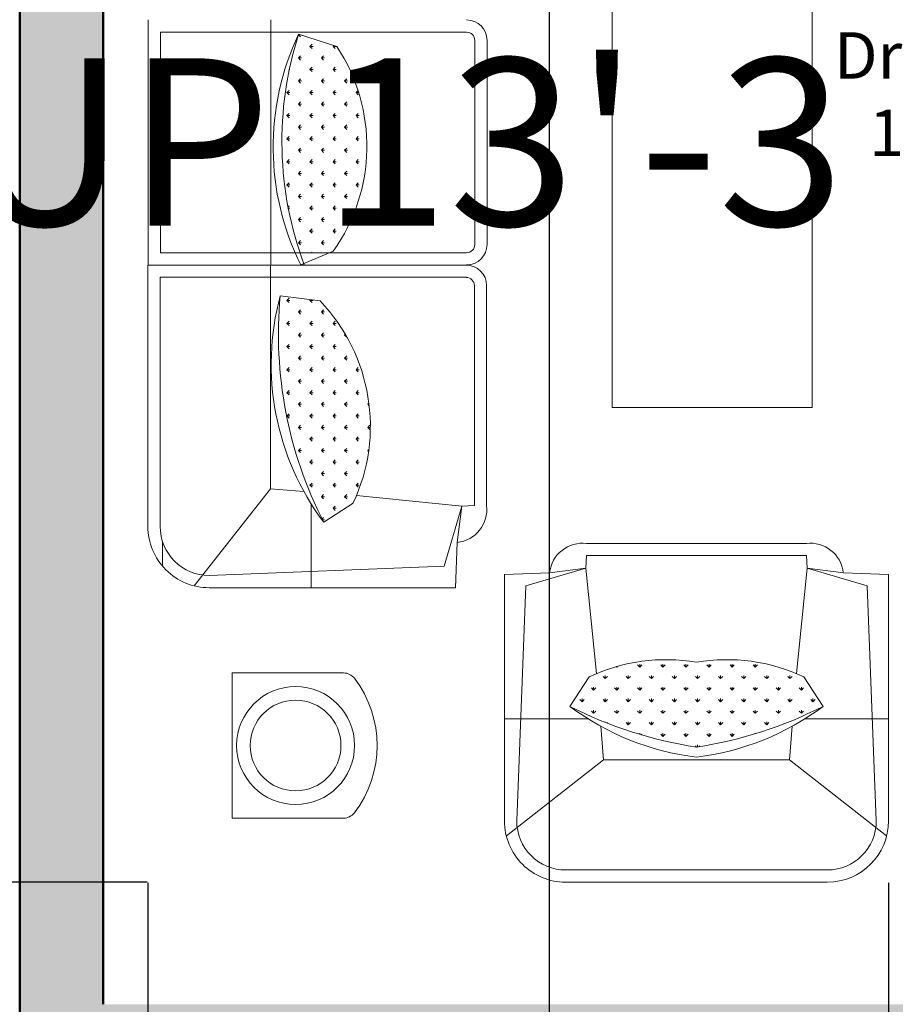
# Model space of a CAD drawing. Units: inches. Extents: x 2796 to 3603, y 978 to 1787.
# Tile 3 of 15: x 3070 to 3165, y 1116 to 1222. Entities that reach past the tile are written whole.
import ezdxf

# ---------------------------------------------------------------- set-up
doc = ezdxf.new("R2010")
doc.units = ezdxf.units.IN
for name, color, linetype, lineweight in [('A-ANNO-DIMS', 7, 'Continuous', 18), ('A-AREA-IDEN', 7, 'Continuous', 18), ('A-WALL-EXTR-PATT', 1, 'Continuous', 13), ('Furniture', 2, 'Continuous', 18), ('Outer Wall', 1, 'Continuous', 50)]:
    doc.layers.add(name, color=color, linetype=linetype, lineweight=lineweight)
doc.styles.get("Standard").update_dxf_attribs({"font": 'arial.ttf'})
doc.dimstyles.get("Standard").update_dxf_attribs({"dimtxt": 18, "dimasz": 12, "dimexe": 0.18, "dimexo": 0.0625, "dimgap": 0.09, "dimtad": 0, "dimtih": 1, "dimtoh": 1, "dimdec": 0, "dimzin": 0, "dimdsep": 46, "dimlunit": 3, "dimtxsty": 'Standard', "dimcen": 0.09, "dimadec": 0, "dimazin": 0, "dimtfac": 1, "dimtdec": 0, "dimtofl": 0, "dimtmove": 0, "dimatfit": 3, "dimfxl": 1, "dimtolj": 1, "dimtzin": 0, "dimarcsym": 0})

# ---------------------------------------------------------------- blocks, each defined once
blk = doc.blocks.new('A$C16A87060')
for p, q in [((2581.2, 1533.8), (2584.8, 1633.4)), ((2584.8, 1633.4), (3128.4, 1633.4)), ((3263.4, 1498.4), (3263.4, 1209.9)), ((1037.3, 1465.2), (2216.9, 1465.2)), ((2216.9, 1465.2), (2216.9, 1024.2)), ((2516.4, 1209.9), (2516.4, 1452.4)), ((2516.4, 1209.9), (2516.4, 967.4)), ((3263.4, 921.4), (3263.4, 1209.9)), ((2216.9, 1024.2), (1037.3, 1024.2)), ((2581.2, 886), (2584.8, 786.4)), ((2584.8, 786.4), (3128.4, 786.4)), ((1407.7, 747.9), (1857.7, 747.9)), ((1948.2, 747), (2433.2, 747)), ((1407.7, 720.9), (1857.7, 720.9)), ((1948.2, 720), (2433.2, 720)), ((2433.2, 720), (2434.6, 692.5)), ((1389.7, 27.9), (1389.7, 702.9)), ((1875.7, 702.9), (1875.7, 27.9)), ((1903.2, 702), (1903.2, 0)), ((1929.7, 702.9), (1929.7, 27)), ((2434.6, 692.5), (2410.9, 460)), ((2514.6, 682.3), (2434.6, 692.5)), ((2566.8, 653.3), (2434.6, 692.5)), ((2514.6, 682.3), (2614.2, 678.6)), ((2614.2, 678.6), (2614.2, 135)), ((1902.7, 667.3), (1903.2, 667.3)), ((2587.2, 135), (2566.8, 653.3)), ((1902.7, 540.3), (1903.2, 540.3)), ((2469.8, 387.7), (2427.5, 452.7)), ((1421.2, 416.7), (1394.2, 332.3)), ((1902.7, 413.3), (1903.2, 413.3)), ((2802.1, 431.6), (2802.1, 185.7)), ((3122.1, 185.7), (3122.1, 431.6)), ((1902.5, 337.3), (1872.5, 408.8)), ((1902.7, 375.2), (1903.2, 375.2)), ((1982.1, 379.8), (1970.5, 291.9)), ((2614.2, 360), (2429.3, 360)), ((2401.8, 343.9), (2396.1, 270)), ((1902.7, 286.3), (1903.2, 286.3)), ((1902.7, 270.9), (1362.7, 270.9)), ((2396.1, 270), (1903.2, 270)), ((2396.1, 270), (2610.1, 101.9)), ((1902.7, 195.2), (1903.2, 195.2)), ((2802.1, 185.7), (3122.1, 185.7)), ((1875.7, 27.9), (1389.7, 27.9)), ((2479.2, 27), (1929.7, 27)), ((2512.6, 32.3), (2566.8, 32.3)), ((1902.7, 0.9), (1362.7, 0.9)), ((2479.2, 0), (1903.2, 0))]:
    blk.add_line(p, q)
at = {"ltscale": 2}
for p, q in [((2903.4, 1633.4), (2903.4, 1448.5)), ((2993.4, 1415.3), (3161.5, 1629.3)), ((3128.4, 1606.4), (2610.2, 1586)), ((2610.2, 1586), (2570.9, 1453.8)), ((2581.2, 1533.8), (2570.9, 1453.8)), ((3236.4, 1498.4), (3236.4, 1209.9)), ((2875.8, 1489), (2810.8, 1446.7)), ((2543.4, 1452.4), (2570.9, 1453.8)), ((2543.4, 1209.9), (2543.4, 1452.4)), ((2570.9, 1453.8), (2803.4, 1430.1)), ((2919.6, 1421), (2993.4, 1415.3)), ((2993.4, 1415.3), (2993.4, 1209.9)), ((2543.4, 1209.9), (2543.4, 967.4)), ((2993.4, 1004.5), (2993.4, 1209.9)), ((3236.4, 921.4), (3236.4, 1209.9)), ((2919.6, 998.8), (2993.4, 1004.5)), ((2993.4, 1004.5), (3161.5, 790.5)), ((2570.9, 966), (2803.4, 989.7)), ((2543.4, 967.4), (2570.9, 966)), ((2581.2, 886), (2570.9, 966)), ((2610.2, 833.8), (2570.9, 966)), ((2875.8, 930.8), (2810.8, 973.1)), ((2903.4, 786.4), (2903.4, 971.3)), ((3128.4, 813.4), (2610.2, 833.8))]:
    blk.add_line(p, q, dxfattribs=at)
at = {"linetype": 'ByBlock'}
for p, q in [((2865.5, 1466.7), (2858.8, 1466.7)), ((2865.5, 1466.7), (2860.7, 1471.5)), ((2865.5, 1466.7), (2860.7, 1462)), ((2840, 1441.3), (2833.3, 1441.3)), ((2840, 1441.3), (2835.3, 1446.1)), ((2840, 1441.3), (2835.3, 1436.5)), ((2891, 1441.3), (2884.2, 1441.3)), ((2891, 1441.3), (2886.2, 1446.1)), ((2891, 1441.3), (2886.2, 1436.5)), ((2814.6, 1415.8), (2807.8, 1415.8)), ((2814.6, 1415.8), (2809.8, 1420.6)), ((2814.6, 1415.8), (2809.8, 1411.1)), ((2865.5, 1415.8), (2858.8, 1415.8)), ((2865.5, 1415.8), (2860.7, 1420.6)), ((2865.5, 1415.8), (2860.7, 1411.1)), ((2840, 1390.4), (2833.3, 1390.4)), ((2840, 1390.4), (2835.3, 1395.1)), ((2840, 1390.4), (2835.3, 1385.6)), ((2891, 1390.4), (2884.2, 1390.4)), ((2891, 1390.4), (2886.2, 1395.1)), ((2891, 1390.4), (2886.2, 1385.6)), ((2814.6, 1364.9), (2809.8, 1369.7)), ((2865.5, 1364.9), (2860.7, 1369.7)), ((2916.4, 1364.9), (2911.6, 1369.7)), ((2814.6, 1364.9), (2807.8, 1364.9)), ((2814.6, 1364.9), (2809.8, 1360.1)), ((2865.5, 1364.9), (2858.8, 1364.9)), ((2865.5, 1364.9), (2860.7, 1360.1)), ((2916.4, 1364.9), (2909.7, 1364.9)), ((2916.4, 1364.9), (2911.6, 1360.1)), ((2789.1, 1339.5), (2782.4, 1339.5)), ((2789.1, 1339.5), (2784.4, 1344.2)), ((2789.1, 1339.5), (2784.4, 1334.7)), ((2840, 1339.5), (2833.3, 1339.5)), ((2840, 1339.5), (2835.3, 1344.2)), ((2840, 1339.5), (2835.3, 1334.7)), ((2891, 1339.5), (2884.2, 1339.5)), ((2891, 1339.5), (2886.2, 1344.2)), ((2891, 1339.5), (2886.2, 1334.7)), ((2936.2, 1339.5), (2935.1, 1339.5)), ((2937.5, 1335.1), (2937.1, 1334.7)), ((2814.6, 1314), (2807.8, 1314)), ((2814.6, 1314), (2809.8, 1318.8)), ((2814.6, 1314), (2809.8, 1309.2)), ((2865.5, 1314), (2858.8, 1314)), ((2865.5, 1314), (2860.7, 1318.8)), ((2865.5, 1314), (2860.7, 1309.2)), ((2916.4, 1314), (2909.7, 1314)), ((2916.4, 1314), (2911.6, 1318.8)), ((2916.4, 1314), (2911.6, 1309.2)), ((2789.1, 1288.5), (2782.4, 1288.5)), ((2789.1, 1288.5), (2784.4, 1293.3)), ((2789.1, 1288.5), (2784.4, 1283.8)), ((2840, 1288.5), (2833.3, 1288.5)), ((2840, 1288.5), (2835.3, 1293.3)), ((2840, 1288.5), (2835.3, 1283.8)), ((2891, 1288.5), (2884.2, 1288.5)), ((2891, 1288.5), (2886.2, 1293.3)), ((2891, 1288.5), (2886.2, 1283.8)), ((2941.9, 1288.5), (2935.1, 1288.5)), ((2941.9, 1288.5), (2937.1, 1293.3)), ((2941.9, 1288.5), (2937.1, 1283.8)), ((2814.6, 1263.1), (2807.8, 1263.1)), ((2814.6, 1263.1), (2809.8, 1267.9)), ((2814.6, 1263.1), (2809.8, 1258.3)), ((2865.5, 1263.1), (2858.8, 1263.1)), ((2865.5, 1263.1), (2860.7, 1267.9)), ((2865.5, 1263.1), (2860.7, 1258.3)), ((2916.4, 1263.1), (2909.7, 1263.1)), ((2916.4, 1263.1), (2911.6, 1267.9)), ((2916.4, 1263.1), (2911.6, 1258.3)), ((2789.1, 1237.6), (2782.4, 1237.6)), ((2789.1, 1237.6), (2784.4, 1242.4)), ((2789.1, 1237.6), (2784.4, 1232.9)), ((2840, 1237.6), (2833.3, 1237.6)), ((2840, 1237.6), (2835.3, 1242.4)), ((2840, 1237.6), (2835.3, 1232.9)), ((2891, 1237.6), (2884.2, 1237.6)), ((2891, 1237.6), (2886.2, 1242.4)), ((2891, 1237.6), (2886.2, 1232.9)), ((2941.9, 1237.6), (2935.1, 1237.6)), ((2941.9, 1237.6), (2937.1, 1242.4)), ((2941.9, 1237.6), (2937.1, 1232.9)), ((2814.6, 1212.2), (2809.8, 1216.9)), ((2865.5, 1212.2), (2860.7, 1216.9)), ((2916.4, 1212.2), (2911.6, 1216.9)), ((2964.7, 1214.8), (2962.6, 1216.9)), ((2814.6, 1212.2), (2807.8, 1212.2)), ((2814.6, 1212.2), (2809.8, 1207.4)), ((2865.5, 1212.2), (2858.8, 1212.2)), ((2865.5, 1212.2), (2860.7, 1207.4)), ((2916.4, 1212.2), (2909.7, 1212.2)), ((2916.4, 1212.2), (2911.6, 1207.4)), ((2965.1, 1212.2), (2960.6, 1212.2)), ((2965.4, 1210.2), (2962.6, 1207.4)), ((2789.1, 1186.7), (2782.4, 1186.7)), ((2789.1, 1186.7), (2784.4, 1191.5)), ((2789.1, 1186.7), (2784.4, 1181.9)), ((2840, 1186.7), (2833.3, 1186.7)), ((2840, 1186.7), (2835.3, 1191.5)), ((2840, 1186.7), (2835.3, 1181.9)), ((2891, 1186.7), (2884.2, 1186.7)), ((2891, 1186.7), (2886.2, 1191.5)), ((2891, 1186.7), (2886.2, 1181.9)), ((2941.9, 1186.7), (2935.1, 1186.7)), ((2941.9, 1186.7), (2937.1, 1191.5)), ((2941.9, 1186.7), (2937.1, 1181.9)), ((2814.6, 1161.3), (2807.8, 1161.3)), ((2814.6, 1161.3), (2809.8, 1166)), ((2814.6, 1161.3), (2809.8, 1156.5)), ((2865.5, 1161.3), (2858.8, 1161.3)), ((2865.5, 1161.3), (2860.7, 1166)), ((2865.5, 1161.3), (2860.7, 1156.5)), ((2916.4, 1161.3), (2909.7, 1161.3)), ((2916.4, 1161.3), (2911.6, 1166)), ((2916.4, 1161.3), (2911.6, 1156.5)), ((2789.1, 1135.8), (2782.4, 1135.8)), ((2789.1, 1135.8), (2784.4, 1140.6)), ((2789.1, 1135.8), (2784.4, 1131)), ((2840, 1135.8), (2833.3, 1135.8)), ((2840, 1135.8), (2835.3, 1140.6)), ((2840, 1135.8), (2835.3, 1131)), ((2891, 1135.8), (2884.2, 1135.8)), ((2891, 1135.8), (2886.2, 1140.6)), ((2891, 1135.8), (2886.2, 1131)), ((2941.9, 1135.8), (2935.1, 1135.8)), ((2941.9, 1135.8), (2937.1, 1140.6)), ((2941.9, 1135.8), (2937.1, 1131)), ((2814.6, 1110.4), (2807.8, 1110.4)), ((2814.6, 1110.4), (2809.8, 1115.1)), ((2814.6, 1110.4), (2809.8, 1105.6)), ((2865.5, 1110.4), (2858.8, 1110.4)), ((2865.5, 1110.4), (2860.7, 1115.1)), ((2865.5, 1110.4), (2860.7, 1105.6)), ((2916.4, 1110.4), (2909.7, 1110.4)), ((2916.4, 1110.4), (2911.6, 1115.1)), ((2916.4, 1110.4), (2911.6, 1105.6)), ((2789.1, 1084.9), (2784.4, 1089.7)), ((2840, 1084.9), (2835.3, 1089.7)), ((2891, 1084.9), (2886.2, 1089.7)), ((2938.5, 1088.2), (2937.1, 1089.7)), ((2789.1, 1084.9), (2782.4, 1084.9)), ((2789.1, 1084.9), (2784.4, 1080.1)), ((2814.6, 1059.4), (2809.8, 1064.2)), ((2840, 1084.9), (2833.3, 1084.9)), ((2840, 1084.9), (2835.3, 1080.1)), ((2865.5, 1059.4), (2860.7, 1064.2)), ((2891, 1084.9), (2884.2, 1084.9)), ((2891, 1084.9), (2886.2, 1080.1)), ((2916.4, 1059.4), (2911.6, 1064.2)), ((2937.5, 1084.9), (2935.1, 1084.9)), ((2814.6, 1059.4), (2807.8, 1059.4)), ((2814.6, 1059.4), (2809.8, 1054.7)), ((2865.5, 1059.4), (2858.8, 1059.4)), ((2865.5, 1059.4), (2860.7, 1054.7)), ((2916.4, 1059.4), (2909.7, 1059.4)), ((2916.4, 1059.4), (2911.6, 1054.7)), ((2789.1, 1034), (2787.5, 1035.6)), ((2789.1, 1034), (2788, 1034)), ((2789.1, 1034), (2788.2, 1033.1)), ((2840, 1034), (2833.3, 1034)), ((2840, 1034), (2835.3, 1038.8)), ((2840, 1034), (2835.3, 1029.2)), ((2891, 1034), (2884.2, 1034)), ((2891, 1034), (2886.2, 1038.8)), ((2891, 1034), (2886.2, 1029.2)), ((2814.6, 1008.5), (2807.8, 1008.5)), ((2814.6, 1008.5), (2809.8, 1013.3)), ((2814.6, 1008.5), (2809.8, 1003.8)), ((2865.5, 1008.5), (2858.8, 1008.5)), ((2865.5, 1008.5), (2860.7, 1013.3)), ((2865.5, 1008.5), (2860.7, 1003.8)), ((2911, 1008.5), (2909.7, 1008.5)), ((2912.5, 1012.4), (2911.6, 1013.3)), ((2840, 983.1), (2833.3, 983.1)), ((2840, 983.1), (2835.3, 987.8)), ((2840, 983.1), (2835.3, 978.3)), ((2891, 983.1), (2884.2, 983.1)), ((2891, 983.1), (2886.2, 987.8)), ((2891, 983.1), (2886.2, 978.3)), ((2865.5, 957.6), (2858.8, 957.6)), ((2865.5, 957.6), (2860.7, 962.4)), ((2865.5, 957.6), (2860.7, 952.8)), ((2209.9, 484.7), (2207.2, 487.4)), ((2209.9, 484.7), (2213.4, 488.1)), ((2209.9, 484.7), (2209.9, 487.7)), ((2260.8, 484.7), (2256.1, 489.5)), ((2260.8, 484.7), (2260.8, 490.6)), ((2260.8, 484.7), (2265.6, 489.5)), ((2311.8, 484.7), (2309.2, 487.3)), ((2311.8, 484.7), (2311.8, 486.9)), ((2311.8, 484.7), (2313.7, 486.7)), ((1522.6, 459.2), (1518.3, 463.5)), ((1522.6, 459.2), (1522.6, 464.9)), ((1522.6, 459.2), (1527.4, 464)), ((1573.5, 459.2), (1568.8, 464)), ((1573.5, 459.2), (1573.5, 466)), ((1573.5, 459.2), (1578.3, 464)), ((1624.5, 459.2), (1619.7, 464)), ((1624.5, 459.2), (1624.5, 466)), ((1624.5, 459.2), (1629.2, 464)), ((1675.4, 459.2), (1670.6, 464)), ((1675.4, 459.2), (1675.4, 466)), ((1675.4, 459.2), (1680.1, 464)), ((1726.3, 459.2), (1721.5, 464)), ((1726.3, 459.2), (1726.3, 466)), ((1726.3, 459.2), (1731, 464)), ((2133.6, 459.2), (2128.8, 464)), ((2133.6, 459.2), (2133.6, 466)), ((2133.6, 459.2), (2138.3, 464)), ((2184.5, 459.2), (2179.7, 464)), ((2184.5, 459.2), (2184.5, 466)), ((2184.5, 459.2), (2189.3, 464)), ((2235.4, 459.2), (2230.6, 464)), ((2235.4, 459.2), (2235.4, 466)), ((2235.4, 459.2), (2240.2, 464)), ((2286.3, 459.2), (2281.5, 464)), ((2286.3, 459.2), (2286.3, 466)), ((2286.3, 459.2), (2291.1, 464)), ((2337.2, 459.2), (2332.4, 464)), ((2337.2, 459.2), (2337.2, 466)), ((2337.2, 459.2), (2342, 464)), ((2388.1, 459.2), (2383.4, 464)), ((2388.1, 459.2), (2388.1, 466)), ((2388.1, 459.2), (2392.9, 464)), ((1497.2, 433.8), (1492.4, 438.5)), ((1497.2, 433.8), (1497.2, 440.5)), ((1497.2, 433.8), (1501.9, 438.5)), ((1548.1, 433.8), (1543.3, 438.5)), ((1548.1, 433.8), (1548.1, 440.5)), ((1548.1, 433.8), (1552.9, 438.5)), ((1599, 433.8), (1594.2, 438.5)), ((1599, 433.8), (1599, 440.5)), ((1599, 433.8), (1603.8, 438.5)), ((1649.9, 433.8), (1645.1, 438.5)), ((1649.9, 433.8), (1649.9, 440.5)), ((1649.9, 433.8), (1654.7, 438.5)), ((1700.8, 433.8), (1696, 438.5)), ((1700.8, 433.8), (1700.8, 440.5)), ((1700.8, 433.8), (1705.6, 438.5)), ((1751.7, 433.8), (1747, 438.5)), ((1751.7, 433.8), (1751.7, 440.5)), ((1751.7, 433.8), (1756.5, 438.5)), ((1802.6, 433.8), (1797.9, 438.5)), ((1802.6, 433.8), (1802.6, 440.5)), ((1802.6, 433.8), (1807.4, 438.5)), ((2057.2, 433.8), (2055.5, 435.4)), ((2057.2, 433.8), (2062, 438.5)), ((2057.2, 433.8), (2057.2, 436.4)), ((2108.1, 433.8), (2103.3, 438.5)), ((2108.1, 433.8), (2108.1, 440.5)), ((2108.1, 433.8), (2112.9, 438.5)), ((2159, 433.8), (2154.3, 438.5)), ((2159, 433.8), (2159, 440.5)), ((2159, 433.8), (2163.8, 438.5)), ((2209.9, 433.8), (2205.2, 438.5)), ((2209.9, 433.8), (2209.9, 440.5)), ((2209.9, 433.8), (2214.7, 438.5)), ((2260.8, 433.8), (2256.1, 438.5)), ((2260.8, 433.8), (2260.8, 440.5)), ((2260.8, 433.8), (2265.6, 438.5)), ((2311.8, 433.8), (2307, 438.5)), ((2311.8, 433.8), (2311.8, 440.5)), ((2311.8, 433.8), (2316.5, 438.5)), ((2362.7, 433.8), (2357.9, 438.5)), ((2362.7, 433.8), (2362.7, 440.5)), ((2362.7, 433.8), (2367.4, 438.5)), ((2413.6, 433.8), (2408.8, 438.5)), ((2413.6, 433.8), (2413.6, 440.5)), ((2413.6, 433.8), (2418.4, 438.5)), ((1420.8, 408.3), (1420.8, 415.1)), ((1420.8, 408.3), (1425.6, 413.1)), ((1471.7, 408.3), (1466.9, 413.1)), ((1471.7, 408.3), (1471.7, 415.1)), ((1471.7, 408.3), (1476.5, 413.1)), ((1522.6, 408.3), (1517.9, 413.1)), ((1522.6, 408.3), (1522.6, 415.1)), ((1522.6, 408.3), (1527.4, 413.1)), ((1573.5, 408.3), (1568.8, 413.1)), ((1573.5, 408.3), (1573.5, 415.1)), ((1573.5, 408.3), (1578.3, 413.1)), ((1624.5, 408.3), (1619.7, 413.1)), ((1624.5, 408.3), (1624.5, 415.1)), ((1624.5, 408.3), (1629.2, 413.1)), ((1675.4, 408.3), (1670.6, 413.1)), ((1675.4, 408.3), (1675.4, 415.1)), ((1675.4, 408.3), (1680.1, 413.1)), ((1726.3, 408.3), (1721.5, 413.1)), ((1726.3, 408.3), (1726.3, 415.1)), ((1726.3, 408.3), (1731, 413.1)), ((1777.2, 408.3), (1772.4, 413.1)), ((1777.2, 408.3), (1777.2, 415.1)), ((1777.2, 408.3), (1782, 413.1)), ((1828.1, 408.3), (1823.3, 413.1)), ((1828.1, 408.3), (1828.1, 415.1)), ((1828.1, 408.3), (1832.9, 413.1)), ((2031.7, 408.3), (2027, 413.1)), ((2031.7, 408.3), (2031.7, 415.1)), ((2031.7, 408.3), (2036.5, 413.1)), ((2082.7, 408.3), (2077.9, 413.1)), ((2082.7, 408.3), (2082.7, 415.1)), ((2082.7, 408.3), (2087.4, 413.1)), ((2133.6, 408.3), (2128.8, 413.1)), ((2133.6, 408.3), (2133.6, 415.1)), ((2133.6, 408.3), (2138.3, 413.1)), ((2184.5, 408.3), (2179.7, 413.1)), ((2184.5, 408.3), (2184.5, 415.1)), ((2184.5, 408.3), (2189.3, 413.1)), ((2235.4, 408.3), (2230.6, 413.1)), ((2235.4, 408.3), (2235.4, 415.1)), ((2235.4, 408.3), (2240.2, 413.1)), ((2286.3, 408.3), (2281.5, 413.1)), ((2286.3, 408.3), (2286.3, 415.1)), ((2286.3, 408.3), (2291.1, 413.1)), ((2337.2, 408.3), (2332.4, 413.1)), ((2337.2, 408.3), (2337.2, 415.1)), ((2337.2, 408.3), (2342, 413.1)), ((2388.1, 408.3), (2383.4, 413.1)), ((2388.1, 408.3), (2388.1, 415.1)), ((2388.1, 408.3), (2392.9, 413.1)), ((2439, 408.3), (2434.3, 413.1)), ((2439, 408.3), (2439, 415.1)), ((2439, 408.3), (2443.8, 413.1)), ((1420.8, 408.3), (1419.1, 410)), ((1446.3, 382.9), (1441.5, 387.6)), ((1446.3, 382.9), (1446.3, 389.6)), ((1446.3, 382.9), (1451, 387.6)), ((1497.2, 382.9), (1492.4, 387.6)), ((1497.2, 382.9), (1497.2, 389.6)), ((1497.2, 382.9), (1501.9, 387.6)), ((1548.1, 382.9), (1543.3, 387.6)), ((1548.1, 382.9), (1548.1, 389.6)), ((1548.1, 382.9), (1552.9, 387.6)), ((1599, 382.9), (1594.2, 387.6)), ((1599, 382.9), (1599, 389.6)), ((1599, 382.9), (1603.8, 387.6)), ((1649.9, 382.9), (1645.1, 387.6)), ((1649.9, 382.9), (1649.9, 389.6)), ((1649.9, 382.9), (1654.7, 387.6)), ((1700.8, 382.9), (1696, 387.6)), ((1700.8, 382.9), (1700.8, 389.6)), ((1700.8, 382.9), (1705.6, 387.6)), ((1751.7, 382.9), (1747, 387.6)), ((1751.7, 382.9), (1751.7, 389.6)), ((1751.7, 382.9), (1756.5, 387.6)), ((1802.6, 382.9), (1797.9, 387.6)), ((1802.6, 382.9), (1802.6, 389.6)), ((1802.6, 382.9), (1807.4, 387.6)), ((1853.6, 382.9), (1848.8, 387.6)), ((1853.6, 382.9), (1853.6, 389.6)), ((1853.6, 382.9), (1858.3, 387.6)), ((2006.3, 382.9), (2001.5, 387.6)), ((2006.3, 382.9), (2006.3, 389.6)), ((2006.3, 382.9), (2011.1, 387.6)), ((2057.2, 382.9), (2052.4, 387.6)), ((2057.2, 382.9), (2057.2, 389.6)), ((2057.2, 382.9), (2062, 387.6)), ((2108.1, 382.9), (2103.3, 387.6)), ((2108.1, 382.9), (2108.1, 389.6)), ((2108.1, 382.9), (2112.9, 387.6)), ((2159, 382.9), (2154.3, 387.6)), ((2159, 382.9), (2159, 389.6)), ((2159, 382.9), (2163.8, 387.6)), ((2209.9, 382.9), (2205.2, 387.6)), ((2209.9, 382.9), (2209.9, 389.6)), ((2209.9, 382.9), (2214.7, 387.6)), ((2260.8, 382.9), (2256.1, 387.6)), ((2260.8, 382.9), (2260.8, 389.6)), ((2260.8, 382.9), (2265.6, 387.6)), ((2311.8, 382.9), (2307, 387.6)), ((2311.8, 382.9), (2311.8, 389.6)), ((2311.8, 382.9), (2316.5, 387.6)), ((2362.7, 382.9), (2357.9, 387.6)), ((2362.7, 382.9), (2362.7, 389.6)), ((2362.7, 382.9), (2367.4, 387.6)), ((2413.6, 382.9), (2408.8, 387.6)), ((2413.6, 382.9), (2413.6, 389.6)), ((2413.6, 382.9), (2418.4, 387.6)), ((2463.1, 384.3), (2459.7, 387.6)), ((2464.5, 385), (2464.5, 389.6)), ((2468.8, 387.2), (2469.3, 387.6)), ((1420.8, 357.4), (1416, 362.2)), ((1420.8, 357.4), (1420.8, 364.2)), ((1420.8, 357.4), (1425.6, 362.2)), ((1471.7, 357.4), (1466.9, 362.2)), ((1471.7, 357.4), (1471.7, 364.2)), ((1471.7, 357.4), (1476.5, 362.2)), ((1522.6, 357.4), (1517.9, 362.2)), ((1522.6, 357.4), (1522.6, 364.2)), ((1522.6, 357.4), (1527.4, 362.2)), ((1573.5, 357.4), (1568.8, 362.2)), ((1573.5, 357.4), (1573.5, 364.2)), ((1573.5, 357.4), (1578.3, 362.2)), ((1624.5, 357.4), (1619.7, 362.2)), ((1624.5, 357.4), (1624.5, 364.2)), ((1624.5, 357.4), (1629.2, 362.2)), ((1675.4, 357.4), (1670.6, 362.2)), ((1675.4, 357.4), (1675.4, 364.2)), ((1675.4, 357.4), (1680.1, 362.2)), ((1726.3, 357.4), (1721.5, 362.2)), ((1726.3, 357.4), (1726.3, 364.2)), ((1726.3, 357.4), (1731, 362.2)), ((1777.2, 357.4), (1772.4, 362.2)), ((1777.2, 357.4), (1777.2, 364.2)), ((1777.2, 357.4), (1782, 362.2)), ((1828.1, 357.4), (1823.3, 362.2)), ((1828.1, 357.4), (1828.1, 364.2)), ((1828.1, 357.4), (1832.9, 362.2)), ((1875.7, 360.7), (1874.2, 362.2)), ((1980.8, 357.4), (1979.3, 358.9)), ((1980.8, 357.4), (1980.8, 364.2)), ((1980.8, 357.4), (1985.6, 362.2)), ((2031.7, 357.4), (2027, 362.2)), ((2031.7, 357.4), (2031.7, 364.2)), ((2031.7, 357.4), (2036.5, 362.2)), ((2082.7, 357.4), (2077.9, 362.2)), ((2082.7, 357.4), (2082.7, 364.2)), ((2082.7, 357.4), (2087.4, 362.2)), ((2133.6, 357.4), (2128.8, 362.2)), ((2133.6, 357.4), (2133.6, 364.2)), ((2133.6, 357.4), (2138.3, 362.2)), ((2184.5, 357.4), (2179.7, 362.2)), ((2184.5, 357.4), (2184.5, 364.2)), ((2184.5, 357.4), (2189.3, 362.2)), ((2235.4, 357.4), (2230.6, 362.2)), ((2235.4, 357.4), (2235.4, 364.2)), ((2235.4, 357.4), (2240.2, 362.2)), ((2286.3, 357.4), (2281.5, 362.2)), ((2286.3, 357.4), (2286.3, 364.2)), ((2286.3, 357.4), (2291.1, 362.2)), ((2337.2, 357.4), (2332.4, 362.2)), ((2337.2, 357.4), (2337.2, 364.2)), ((2337.2, 357.4), (2342, 362.2)), ((2388.1, 357.4), (2383.4, 362.2)), ((2388.1, 357.4), (2388.1, 364.2)), ((2388.1, 357.4), (2392.9, 362.2)), ((1395.3, 331.9), (1394.4, 332.9)), ((1395.3, 331.9), (1400.1, 336.7)), ((1395.3, 331.9), (1395.3, 336)), ((1446.3, 331.9), (1441.5, 336.7)), ((1446.3, 331.9), (1446.3, 338.7)), ((1446.3, 331.9), (1451, 336.7)), ((1497.2, 331.9), (1492.4, 336.7)), ((1497.2, 331.9), (1497.2, 338.7)), ((1497.2, 331.9), (1501.9, 336.7)), ((1548.1, 331.9), (1543.3, 336.7)), ((1548.1, 331.9), (1548.1, 338.7)), ((1548.1, 331.9), (1552.9, 336.7)), ((1599, 331.9), (1594.2, 336.7)), ((1599, 331.9), (1599, 338.7)), ((1599, 331.9), (1603.8, 336.7)), ((1649.9, 331.9), (1645.1, 336.7)), ((1649.9, 331.9), (1649.9, 338.7)), ((1649.9, 331.9), (1654.7, 336.7)), ((1700.8, 331.9), (1696, 336.7)), ((1700.8, 331.9), (1700.8, 338.7)), ((1700.8, 331.9), (1705.6, 336.7)), ((1751.7, 331.9), (1747, 336.7)), ((1751.7, 331.9), (1751.7, 338.7)), ((1751.7, 331.9), (1756.5, 336.7)), ((1802.6, 331.9), (1797.9, 336.7)), ((1802.6, 331.9), (1802.6, 338.7)), ((1802.6, 331.9), (1807.4, 336.7)), ((1853.6, 331.9), (1848.8, 336.7)), ((1853.6, 331.9), (1853.6, 338.7)), ((1853.6, 331.9), (1858.3, 336.7)), ((2006.3, 331.9), (2001.5, 336.7)), ((2006.3, 331.9), (2006.3, 338.7)), ((2006.3, 331.9), (2011.1, 336.7)), ((2057.2, 331.9), (2052.4, 336.7)), ((2057.2, 331.9), (2057.2, 338.7)), ((2057.2, 331.9), (2062, 336.7)), ((2108.1, 331.9), (2103.3, 336.7)), ((2108.1, 331.9), (2108.1, 338.7)), ((2108.1, 331.9), (2112.9, 336.7)), ((2159, 331.9), (2154.3, 336.7)), ((2159, 331.9), (2159, 338.7)), ((2159, 331.9), (2163.8, 336.7)), ((2209.9, 331.9), (2205.2, 336.7)), ((2209.9, 331.9), (2209.9, 338.7)), ((2209.9, 331.9), (2214.7, 336.7)), ((2260.8, 331.9), (2256.1, 336.7)), ((2260.8, 331.9), (2260.8, 338.7)), ((2260.8, 331.9), (2265.6, 336.7)), ((2311.8, 331.9), (2307, 336.7)), ((2311.8, 331.9), (2311.8, 338.7)), ((2311.8, 331.9), (2316.5, 336.7)), ((1471.7, 311.9), (1471.7, 313.2)), ((1476.2, 311), (1476.5, 311.3)), ((1522.6, 306.5), (1517.9, 311.3)), ((1522.6, 306.5), (1522.6, 313.2)), ((1522.6, 306.5), (1527.4, 311.3)), ((1573.5, 306.5), (1568.8, 311.3)), ((1573.5, 306.5), (1573.5, 313.2)), ((1573.5, 306.5), (1578.3, 311.3)), ((1624.5, 306.5), (1619.7, 311.3)), ((1624.5, 306.5), (1624.5, 313.2)), ((1624.5, 306.5), (1629.2, 311.3)), ((1675.4, 306.5), (1670.6, 311.3)), ((1675.4, 306.5), (1675.4, 313.2)), ((1675.4, 306.5), (1680.1, 311.3)), ((1726.3, 306.5), (1721.5, 311.3)), ((1726.3, 306.5), (1726.3, 313.2)), ((1726.3, 306.5), (1731, 311.3)), ((1774.6, 309.1), (1772.4, 311.3)), ((1777.2, 309.5), (1777.2, 313.2)), ((1781, 310.3), (1782, 311.3)), ((1980.8, 306.5), (1976.1, 311.3)), ((1980.8, 306.5), (1980.8, 313.2)), ((1980.8, 306.5), (1985.6, 311.3)), ((2031.7, 306.5), (2027, 311.3)), ((2031.7, 306.5), (2031.7, 313.2)), ((2031.7, 306.5), (2036.5, 311.3)), ((2082.7, 306.5), (2077.9, 311.3)), ((2082.7, 306.5), (2082.7, 313.2)), ((2082.7, 306.5), (2087.4, 311.3)), ((2133.6, 306.5), (2128.8, 311.3)), ((2133.6, 306.5), (2133.6, 313.2)), ((2133.6, 306.5), (2138.3, 311.3)), ((2184.5, 306.5), (2179.7, 311.3)), ((2184.5, 306.5), (2184.5, 313.2)), ((2184.5, 306.5), (2189.3, 311.3)), ((2235.4, 306.5), (2230.6, 311.3)), ((2235.4, 306.5), (2235.4, 313.2)), ((2235.4, 306.5), (2240.2, 311.3))]:
    blk.add_line(p, q, dxfattribs=at)
for radius in [130, 100]:
    blk.add_circle((2962.1, 325.7), radius)
for centre, radius, start, end in [((3128.4, 1498.4), 135, 0, 90), ((2589.4, 1460.8), 73.4, 96.4251, 186.5821), ((2589.4, 959), 73.4, 173.4179, 263.5749), ((3128.4, 921.4), 135, 270, 0), ((1407.7, 702.9), 45, 90, 180), ((1857.7, 702.9), 45, 0, 90), ((1948.2, 702), 45, 90, 180), ((2441.6, 674.1), 73.4, 6.4251, 96.5821), ((1407.7, 702.9), 18, 90, 180), ((1857.7, 702.9), 18, 0, 90), ((1948.2, 702), 18, 90, 180), ((2962.1, 262.4), 243.3, 52.4557, 127.5443), ((1641.1, 84.6), 398.3, 54.4888, 123.508), ((2257.8, 92.3), 398.3, 64.7866, 133.8058), ((2832.1, 431.6), 30, 127.5443, 180), ((3092.1, 431.6), 30, 0, 52.4557), ((2121.7, 853.2), 581.3, 254.928, 306.7929), ((2055.5, 1197.9), 910, 264.6406, 297.0804), ((1300.3, 2138.7), 1869.7, 288.7972, 288.812), ((1630.3, 1071.1), 775.6, 252.2742, 290.5658), ((1643.2, 857.5), 581.3, 244.6302, 296.4951), ((1300.3, 2138.7), 1892.2, 288.5655, 288.5801), ((2479.2, 135), 135, 270, 0), ((2479.2, 135), 108, 270, 0)]:
    blk.add_arc(centre, radius, start, end)
at = {"ltscale": 2}
for centre, radius, start, end in [((3128.4, 1498.4), 108, 0, 90), ((2065.5, 1074.7), 910, 8.543, 27.0804), ((2410.3, 1140.9), 581.3, 6.8212, 36.7929), ((3171.1, 1277), 398.3, 154.7866, 189.6954), ((3171.1, 1142.8), 398.3, 170.3046, 205.2134), ((2410.3, 1278.9), 581.3, 323.2071, 353.1788), ((2065.5, 1345.1), 910, 332.9196, 351.457), ((3128.4, 921.4), 108, 270, 0)]:
    blk.add_arc(centre, radius, start, end, dxfattribs=at)
blk = doc.blocks.new('*D12')
at = {"layer": 'A-ANNO-DIMS', "color": 0, "lineweight": -2, "transparency": 16777216}
for p, q in [((3070.18, 1736.68), (3041.33, 1736.68)), ((3041.51, 1724.68), (3041.51, 1391.96)), ((3041.51, 1040.68), (3041.51, 1373.4)), ((3070.18, 1028.68), (3041.33, 1028.68))]:
    blk.add_line(p, q, dxfattribs=at)
at = {"layer": 'A-ANNO-DIMS', "color": 0, "transparency": 16777216}
for points in [[(3039.51, 1724.68), (3043.51, 1724.68), (3041.51, 1736.68)], [(3039.51, 1040.68), (3043.51, 1040.68), (3041.51, 1028.68)]]:
    blk.add_solid(points, dxfattribs=at)
at = {"layer": 'Defpoints', "color": 0, "transparency": 16777216}
for p in [(3041.51, 1736.68), (3070.25, 1736.68), (3070.25, 1028.68)]:
    blk.add_point(p, dxfattribs=at)
at = {"layer": 'A-ANNO-DIMS', "color": 0, "transparency": 16777216, "insert": (3041.51, 1382.68), "char_height": 18, "attachment_point": 5}
blk.add_mtext("\\A1;59'", dxfattribs=at)
blk = doc.blocks.new('*D30')
at = {"layer": 'A-ANNO-DIMS', "color": 0, "lineweight": -2, "transparency": 16777216}
for p, q in [((3083.98, 1288.1), (3059.97, 1288.1)), ((3060.15, 1276.1), (3060.15, 1217.86)), ((3060.15, 1140.81), (3060.15, 1199.05)), ((3083.98, 1128.81), (3059.97, 1128.81))]:
    blk.add_line(p, q, dxfattribs=at)
at = {"layer": 'A-ANNO-DIMS', "color": 0, "transparency": 16777216}
for points in [[(3058.15, 1276.1), (3062.15, 1276.1), (3060.15, 1288.1)], [(3058.15, 1140.81), (3062.15, 1140.81), (3060.15, 1128.81)]]:
    blk.add_solid(points, dxfattribs=at)
at = {"layer": 'Defpoints', "color": 0, "transparency": 16777216}
for p in [(3084.05, 1288.1), (3060.15, 1128.81), (3084.05, 1128.81)]:
    blk.add_point(p, dxfattribs=at)
at = {"layer": 'A-ANNO-DIMS', "color": 0, "transparency": 16777216, "insert": (3060.15, 1208.46), "char_height": 18, "attachment_point": 5}
blk.add_mtext('\\A1;SEATING GROUP 13\'-3 1/2"', dxfattribs=at)
blk = doc.blocks.new('*D31')
at = {"layer": 'A-ANNO-DIMS', "color": 0, "lineweight": -2, "transparency": 16777216}
for p, q in [((3084.05, 1128.75), (3084.05, 1104.74)), ((3163.77, 1128.75), (3163.77, 1104.74)), ((3096.05, 1104.92), (3151.77, 1104.92)), ((3163.77, 1104.92), (3175.77, 1104.92))]:
    blk.add_line(p, q, dxfattribs=at)
at = {"layer": 'A-ANNO-DIMS', "color": 0, "transparency": 16777216}
for points in [[(3096.05, 1106.92), (3096.05, 1102.92), (3084.05, 1104.92)], [(3151.77, 1106.92), (3151.77, 1102.92), (3163.77, 1104.92)]]:
    blk.add_solid(points, dxfattribs=at)
at = {"layer": 'Defpoints', "color": 0, "transparency": 16777216}
for p in [(3084.05, 1128.81), (3163.77, 1128.81), (3163.77, 1104.92)]:
    blk.add_point(p, dxfattribs=at)
at = {"layer": 'A-ANNO-DIMS', "color": 0, "transparency": 16777216, "insert": (3220.81, 1104.92), "char_height": 18, "attachment_point": 5}
blk.add_mtext('\\A1;6\'-7 1/2"', dxfattribs=at)
blk = doc.blocks.new('*D51')
at = {"layer": 'A-ANNO-DIMS', "color": 0, "lineweight": -2, "transparency": 16777216}
for p, q in [((3127.245499, 1431.61284), (3127.245499, 989.79534)), ((3199.245499, 1431.61284), (3199.245499, 989.79534)), ((3115.245499, 989.97534), (3103.245499, 989.97534)), ((3211.245499, 989.97534), (3223.245499, 989.97534))]:
    blk.add_line(p, q, dxfattribs=at)
at = {"layer": 'A-ANNO-DIMS', "color": 0, "transparency": 16777216}
for points in [[(3115.245499, 991.97534), (3115.245499, 987.97534), (3127.245499, 989.97534)], [(3211.245499, 991.97534), (3211.245499, 987.97534), (3199.245499, 989.97534)]]:
    blk.add_solid(points, dxfattribs=at)
at = {"layer": 'Defpoints', "color": 0, "transparency": 16777216}
for p in [(3127.245499, 1431.67534), (3199.245499, 1431.67534), (3199.245499, 989.97534)]:
    blk.add_point(p, dxfattribs=at)
at = {"layer": 'A-ANNO-DIMS', "color": 0, "transparency": 16777216, "insert": (3163.245499, 989.97534), "char_height": 18, "attachment_point": 5}
blk.add_mtext('\\A1;6\'-0"', dxfattribs=at)

msp = doc.modelspace()

# ---------------------------------------------------------------- hatches: boundary and pattern name
at = {"layer": 'A-WALL-EXTR-PATT'}
h = msp.add_hatch(color=256, dxfattribs=at)
h.dxf.hatch_style = 1
h.paths.add_polyline_path([(3424.25, 1736.68), (3070.25, 1736.68), (3070.25, 1106.68), (3227.25, 1106.68), (3227.25, 1115.68), (3226.75, 1115.68), (3223.75, 1115.68), (3079.25, 1115.68), (3079.25, 1727.68), (3127.25, 1727.68), (3415.25, 1727.68), (3415.25, 1188.68), (3424.25, 1188.68)])
h.paths.add_polyline_path([(3291.25, 1032.68), (3074.25, 1032.68), (3074.25, 1106.68), (3070.25, 1106.68), (3070.25, 1028.68), (3291.25, 1028.68)])
h.paths.add_polyline_path([(3291.25, 1115.68), (3281.25, 1115.68), (3281.25, 1106.68), (3291.25, 1106.68)], flags=17)
h.paths.add_polyline_path([(3301.25, 1037.68), (3291.25, 1037.68), (3291.25, 1028.68), (3301.25, 1028.68)])
h.paths.add_polyline_path([(3424.25, 1037.68), (3414.25, 1037.68), (3414.25, 1028.68), (3424.25, 1028.68)])
h.paths.add_polyline_path([(3424.25, 1188.68), (3420.25, 1188.68), (3420.25, 1037.68), (3424.25, 1037.68)])

# ---------------------------------------------------------------- linework, layer by layer
at = {"layer": 'Outer Wall'}
for p, q in [((3070.25, 1028.68), (3070.25, 1736.68)), ((3079.25, 1115.68), (3079.25, 1727.68))]:
    msp.add_line(p, q, dxfattribs=at)

# ---------------------------------------------------------------- block references
at = {"layer": 'Furniture', "xscale": 0.0488098627676315, "yscale": 0.0488098627676315, "zscale": 0.0488098627676315, "rotation": 270}
msp.add_blockref('A$C16A87060', (3084.05, 1288.1), dxfattribs=at)

# ---------------------------------------------------------------- texts
at = {"layer": 'A-AREA-IDEN', "insert": (3209.15, 1220.27), "char_height": 5, "attachment_point": 3}
msp.add_mtext_dynamic_manual_height_columns('\\pxqc;{\\fTimes New Roman|b0|i0|c0|p18;Drawing Room\\P12\'0" x 16\'0"}', width=55.5021, gutter_width=12.5, heights=[0], dxfattribs=at)

# ---------------------------------------------------------------- dimensions: what is measured, and where the dimension line sits
at = {"layer": 'A-ANNO-DIMS'}
dim = msp.add_linear_dim(base=(3041.51, 1736.68), p1=(3070.25, 1028.68), p2=(3070.25, 1736.68), angle=90, dimstyle='Standard', override={"dimclrd": 0, "dimclre": 0, "dimclrt": 0}, dxfattribs=at)
dim.commit()
dim.dimension.update_dxf_attribs({"geometry": '*D12', "text_midpoint": (3041.51, 1382.68)})
for base, p1, p2, picture, middle in [((3199.25, 989.98), (3127.25, 1431.68), (3199.25, 1431.68), '*D51', (3163.25, 989.98)), ((3163.77, 1104.92), (3084.05, 1128.81), (3163.77, 1128.81), '*D31', (3220.81, 1104.92))]:
    dim = msp.add_linear_dim(base=base, p1=p1, p2=p2, dimstyle='Standard', override={"dimdec": 1, "dimlfac": 1, "dimrnd": 0, "dimzin": 1, "dimdsep": 46, "dimlunit": 4, "dimfrac": 2}, dxfattribs=at)
    dim.commit()
    dim.dimension.update_dxf_attribs({"geometry": picture, "text_midpoint": middle})
dim = msp.add_linear_dim(base=(3060.15, 1128.81), p1=(3084.05, 1288.1), p2=(3084.05, 1128.81), angle=270, text='SEATING GROUP <>', dimstyle='Standard', override={"dimdec": 1, "dimlfac": 1, "dimrnd": 0, "dimzin": 1, "dimdsep": 46, "dimlunit": 4, "dimfrac": 2}, dxfattribs=at)
dim.commit()
dim.dimension.update_dxf_attribs({"geometry": '*D30', "text_midpoint": (3060.15, 1208.46)})

doc.saveas('drawing.dxf')
